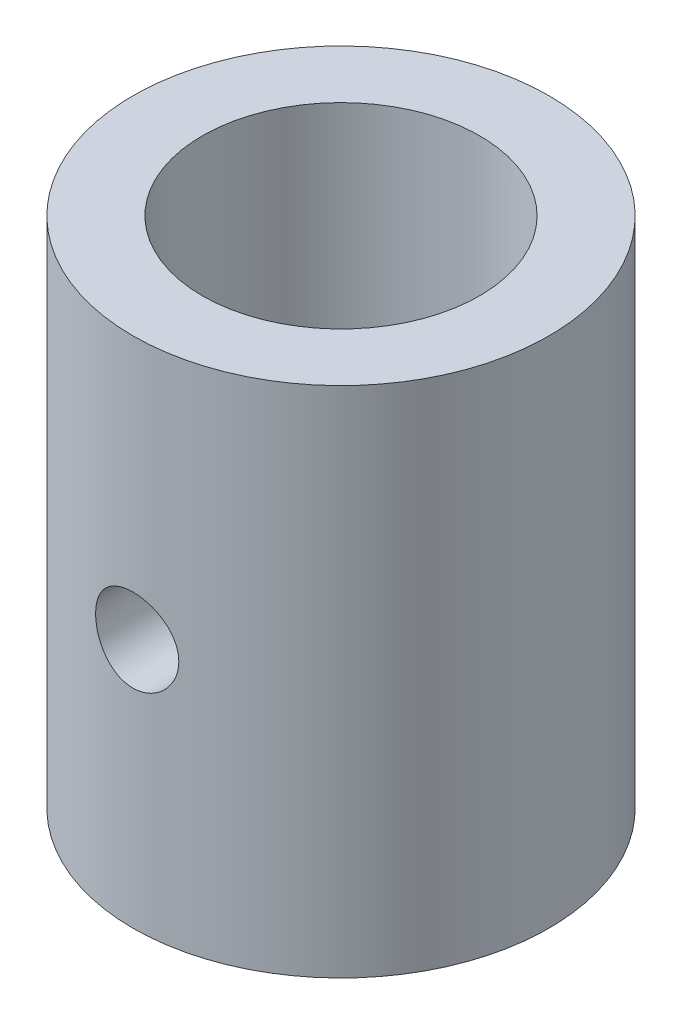
from build123d import *

# Parameters (mm, degrees)
BUSH_RING_PROFILE_SKETCH_R   = 15
BUSH_RING_PROFILE_SKETCH_R_2 = 10
BUSH_BODY_30X_20X37_DEPTH    = 18.5
CROSS_HOLE_SKETCH_R          = 3
CROSS_HOLE_6_DEPTH           = 18.5


with BuildPart() as part:
    # Bush Ring Profile Sketch → Bush Body Ø30xØ20x37 (new, symmetric)
    with BuildSketch(Plane(origin=(0, 0, 0), x_dir=(1, 0, 0), z_dir=(0, 1, 0))):
        with Locations(Location((0, 0, 0), (0, 0, 270))):
            Circle(BUSH_RING_PROFILE_SKETCH_R)
        with Locations(Location((0, 0, 0), (0, 0, 270))):
            Circle(BUSH_RING_PROFILE_SKETCH_R_2, mode=Mode.SUBTRACT)
    extrude(amount=BUSH_BODY_30X_20X37_DEPTH, both=True)

    # Cross Hole Sketch → Cross Hole Ø6 (cut, symmetric)
    with BuildSketch(Plane.XY):
        with Locations((0, -0.5)):
            Circle(CROSS_HOLE_SKETCH_R)
    extrude(amount=CROSS_HOLE_6_DEPTH, both=True, mode=Mode.SUBTRACT)


solid = part.part
